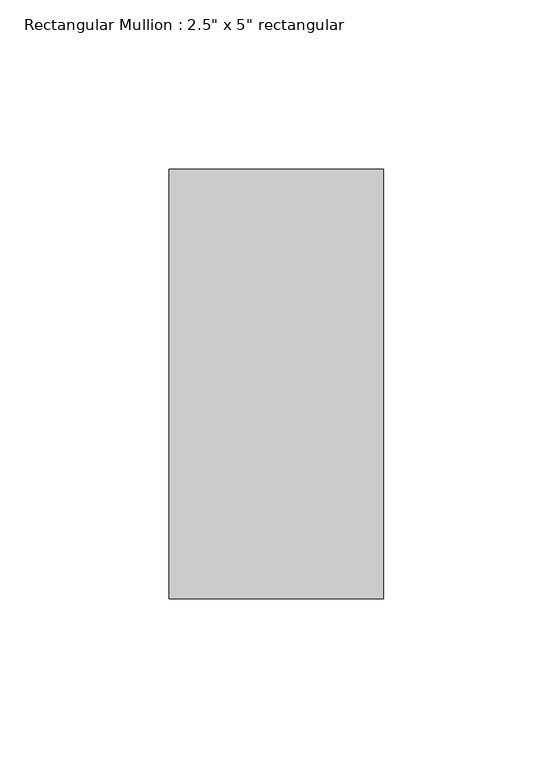
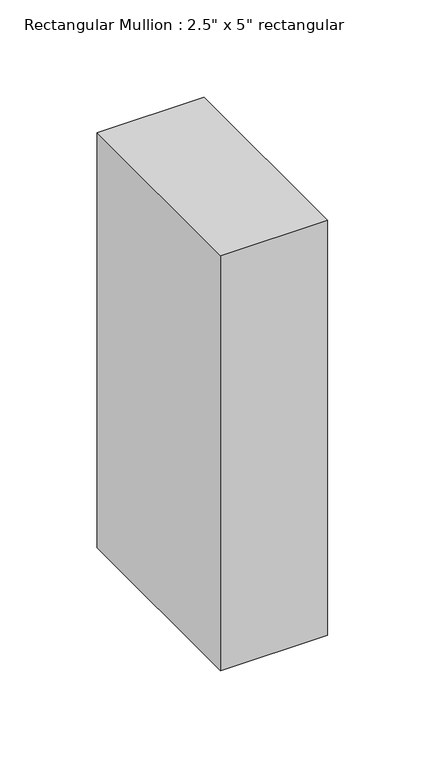
"""IFC4 building model written with IfcOpenShell, lengths in millimetres: member geometry."""

from ifc_helpers import new_model, si_unit, frame, origin, place, context, project, spatial, polyline, outline, extrude, source, transform, mapped, element, save


def member_4adcbd6e(model_context):
    return source(origin(), model_context, "Body", "SweptSolid", [
        extrude(outline(polyline([(0.0, 63.5), (0.0, -63.5), (-63.5, -63.5), (-63.5, 63.5), (0.0, 63.5)])), frame((0.0, 0.0, -260.35), z_axis=(0.0, 0.0, 1.0), x_axis=(1.0, 0.0, 0.0)), (0.0, 0.0, 1.0), 260.35),
    ])


if __name__ == "__main__":
    model = new_model("IFC4")
    model_context = context("Model", 3, world=origin())
    ifc_project = project(units=[si_unit("LENGTHUNIT", "METRE", prefix="MILLI")], contexts=[model_context])
    site = spatial("IfcSite", under=ifc_project)
    building = spatial("IfcBuilding", under=site)
    placement = place(None, origin())
    member_shape = member_4adcbd6e(model_context)
    element("IfcMember", 1, ObjectType="Rectangular Mullion : 2.5\" x 5\" rectangular", at=placement, inside=building, context=model_context, shape_type="MappedRepresentation", body=[
        mapped(member_shape, transform((0.0, 0.0, 0.0), x_axis=(1.0, 0.0, 0.0), y_axis=(0.0, 1.0, 0.0), z_axis=(0.0, 0.0, 1.0))),
    ])
    save(model, "model.ifc")

# Revit data of these elements
# Type "Rectangular Mullion : 2.5\" x 5\" rectangular"
#   built-in parameter 1007304 = 0.416667 (stored number, unit not read)
#   built-in parameter 1007301 = 0.104167 (stored number, unit not read)
#   built-in parameter 1007300 = 0.104167 (stored number, unit not read)
